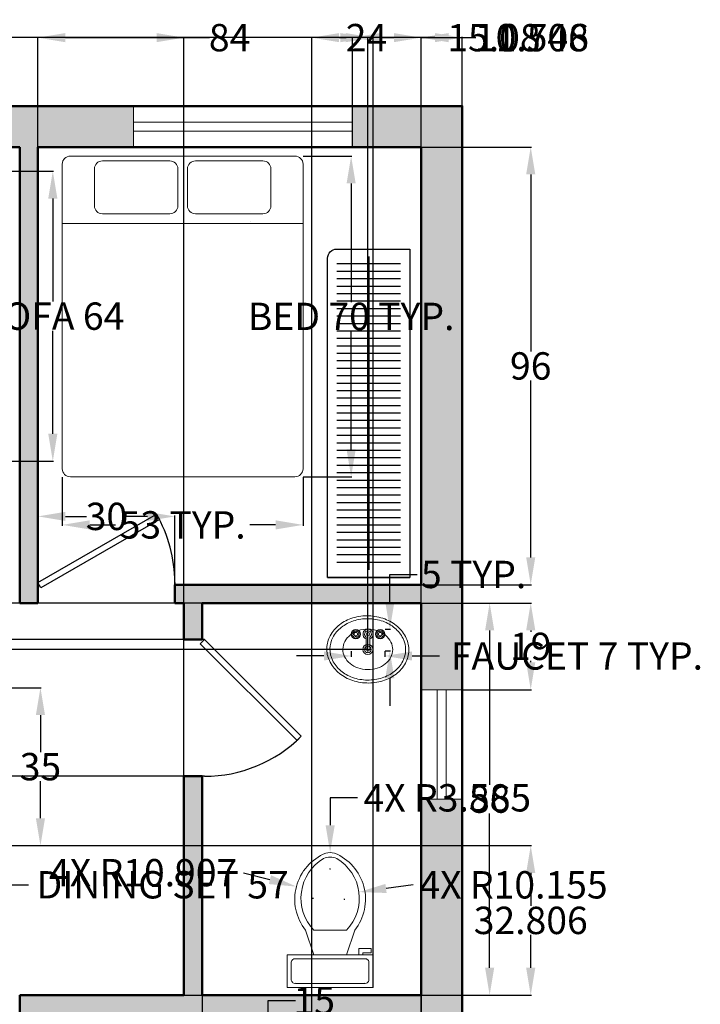
# Model space of a CAD drawing. Units: inches. Extents: x -11 to 341, y -300 to 41.
# Tile 5 of 5: x 192 to 341, y -178 to 38. Entities that reach past the tile are written whole.
import ezdxf

# ---------------------------------------------------------------- set-up
doc = ezdxf.new("R2010")
doc.units = ezdxf.units.IN
doc.header["$MEASUREMENT"] = 0
for name, color, linetype, lineweight in [('A-ANNO-DIMS', 2, 'Continuous', 18), ('A-DOOR', 3, 'Continuous', 25), ('A-FLOR-CASE', 8, 'Continuous', 25), ('A-FLOR-FIXT', 9, 'Continuous', 18), ('A-FURN', 8, 'Continuous', 18), ('A-GLAZ', 4, 'Continuous', 18), ('A-WALL', 7, 'Continuous', 50), ('A-WALL-PATT', 251, 'Continuous', 13)]:
    doc.layers.add(name, color=color, linetype=linetype, lineweight=lineweight)
doc.styles.get("Standard").update_dxf_attribs({"font": 'arial.ttf'})
doc.dimstyles.get("Standard").update_dxf_attribs({"dimtxt": 6, "dimasz": 6, "dimexe": 0.18, "dimexo": 0.0625, "dimgap": 0.09, "dimtad": 0, "dimtih": 1, "dimtoh": 1, "dimdec": 0, "dimzin": 0, "dimdsep": 46, "dimlunit": 4, "dimtxsty": 'Standard', "dimcen": 0.09, "dimadec": 0, "dimazin": 0, "dimtfac": 1, "dimtdec": 0, "dimtofl": 0, "dimtmove": 0, "dimatfit": 3, "dimfxl": 1, "dimtolj": 1, "dimtzin": 0, "dimarcsym": 0})

# ---------------------------------------------------------------- blocks, each defined once
blk = doc.blocks.new('*U2')
for p, q in [((0, 0), (0, -6)), ((40, 0), (40, -6))]:
    blk.add_line(p, q)
blk.add_lwpolyline([(0, 0), (34.64, 20), (35.52, 18.48), (0.87, -1.52)], close=True)
blk.add_arc((0, 0), 40, 0, 30)
blk = doc.blocks.new('*U14')
for p, q in [((0, 0), (0, -6)), ((40, 0), (40, -6))]:
    blk.add_line(p, q)
blk.add_lwpolyline([(0, 0), (28.28, 28.28), (29.52, 27.05), (1.24, -1.24)], close=True)
blk.add_arc((0, 0), 40, 0, 45)
blk = doc.blocks.new('Bed - Queen')
for p, q in [((2, 0), (57.99999, 0)), ((0, -78.00003), (0, -2)), ((9.99999, -1.2), (26.79998, -1.2)), ((33.19999, -1.2), (49.99999, -1.2)), ((59.99999, -2), (59.99999, -78.00003)), ((7.99999, -12.4), (7.99999, -3.2)), ((28.79998, -3.2), (28.79998, -12.4)), ((31.19999, -12.4), (31.19999, -3.2)), ((51.99999, -3.2), (51.99999, -12.4)), ((9.99999, -14.4), (26.79998, -14.4)), ((33.19999, -14.4), (49.99999, -14.4)), ((59.99999, -16.8), (0, -16.8)), ((46.8, -16.4), (46.79936, -16.4)), ((57.99999, -80.00003), (2, -80.00003))]:
    blk.add_line(p, q)
for centre, start, end in [((2, -2), 90, 180), ((57.99999, -2), 0, 90), ((9.99999, -3.2), 90, 180), ((26.79998, -3.2), 0, 90), ((33.19999, -3.2), 90, 180), ((49.99999, -3.2), 0, 90), ((9.99999, -12.4), 180, 270), ((26.79998, -12.4), 270, 0), ((33.19999, -12.4), 180, 270), ((49.99999, -12.4), 270, 0), ((2, -78.00003), 180, 270), ((57.99999, -78.00003), 270, 0)]:
    blk.add_arc(centre, 2, start, end)
blk = doc.blocks.new('Toilet - top')
for p, q in [((9.5, -6), (9.5, -2)), ((-10, -8.5), (-8, -8.5)), ((-10, -9.5), (-10, -8.5)), ((-7, -9.5), (-10, -9.5)), ((-8, -8.5), (-8, -8)), ((-7, -8), (-7, -9.5)), ((-4, -8), (-6, -14)), ((4, -8), (6, -14)), ((4, -14), (-4, -14))]:
    blk.add_line(p, q)
blk.add_lwpolyline([(10.5, -8), (10.5, 0), (-10.5, 0), (-10.5, -8)], close=True)
for points in [[(-9.5, -2), (-9.5, -6)], [(8.5, -1), (-8.5, -1)], [(-8.5, -7), (8.5, -7)]]:
    blk.add_lwpolyline(points)
for centre, radius, start, end in [((-8.62, -1.88), 0.884, 81.8699, 188.1301), ((8.62, -1.88), 0.884, 351.8699, 98.1301), ((-8.62, -6.12), 0.884, 171.8699, 278.1301), ((8.62, -6.12), 0.884, 261.8699, 8.1301), ((3.52, -21.58), 12.17, 141.4691, 247.9714), ((4.2, -21.82), 11.33, 136.3677, 238.9468), ((-3.52, -21.58), 12.17, 292.0284, 38.5307), ((-4.2, -21.82), 11.33, 301.053, 43.6321), ((0, -27.88), 4, 245.7318, 294.2682), ((0, -29), 4, 254.8605, 285.1395)]:
    blk.add_arc(centre, radius, start, end)
blk = doc.blocks.new('Sink - Oval top')
for p, q in [((-1, 0), (1, 0)), ((0, 1), (0, -1))]:
    blk.add_line(p, q)
for points in [[(-12.23, 0.39, 0.117634), (-11.46, -3.36, 0.104469), (-8.88, -6.8, 0.090016), (-5.08, -9.07, 0.08192), (-0.32, -10.02, 0.08192), (4.49, -9.38, 0.090016), (8.42, -7.36, 0.104469), (11.22, -4.09, 0.117634), (12.23, -0.39, 0.117634), (11.46, 3.36, 0.104469), (8.88, 6.8, 0.090016), (5.08, 9.07, 0.08192), (0.32, 10.02, 0.08192), (-4.49, 9.38, 0.090016), (-8.42, 7.36, 0.104469), (-11.22, 4.09, 0.117634)], [(-11.29, 0.16, 0.118622), (-10.52, -3.25, 0.104678), (-8.07, -6.36, 0.089562), (-4.54, -8.37, 0.081185), (-0.13, -9.15, 0.081185), (4.3, -8.49, 0.089562), (7.89, -6.58, 0.104678), (10.42, -3.55, 0.118622), (11.29, -0.16, 0.118622), (10.52, 3.25, 0.104678), (8.07, 6.36, 0.089562), (4.54, 8.37, 0.081185), (0.13, 9.15, 0.081185), (-4.3, 8.49, 0.089562), (-7.89, 6.58, 0.104678), (-10.42, 3.55, 0.118622)], [(-7.42, 0.08, 0.118283), (-6.91, -2.17, 0.104607), (-5.29, -4.21, 0.089718), (-2.97, -5.53, 0.081436), (-0.07, -6.04, 0.081436), (2.84, -5.59, 0.089718), (5.2, -4.33, 0.104607), (6.86, -2.32, 0.118283), (7.42, -0.08, 0.118283), (6.91, 2.17, 0.104607), (5.29, 4.21, 0.089718), (2.97, 5.53, 0.081436), (0.07, 6.04, 0.081436), (-2.84, 5.59, 0.089718), (-5.2, 4.33, 0.104607), (-6.86, 2.32, 0.118283)]]:
    blk.add_lwpolyline(points, format="xyb", close=True)
for radius in [1.5, 1]:
    blk.add_circle((0, 0), radius)
blk = doc.blocks.new('Faucet - Bathroom top')
for p, q in [((-4.107, 0.125), (-4.375, 0.125)), ((-3.75, 0.4788), (-3.75, 0.75)), ((-3.5, 0.482), (-3.5, 0.75)), ((-3.1461, 0.125), (-2.875, 0.125)), ((3.143, 0.125), (2.875, 0.125)), ((3.5, 0.4788), (3.5, 0.75)), ((3.75, 0.482), (3.75, 0.75)), ((4.1039, 0.125), (4.375, 0.125)), ((-4.1039, -0.125), (-4.375, -0.125)), ((-3.75, -0.4821), (-3.75, -0.75)), ((-3.5, -0.4789), (-3.5, -0.75)), ((-3.143, -0.125), (-2.875, -0.125)), ((-0.5, -0.8639), (-0.5, -4.5)), ((0.5, -4.5), (0.5, -0.8631)), ((3.1461, -0.125), (2.875, -0.125)), ((3.5, -0.4821), (3.5, -0.75)), ((3.75, -0.4789), (3.75, -0.75)), ((4.107, -0.125), (4.375, -0.125))]:
    blk.add_line(p, q)
for centre, radius in [((-3.625, 0), 1.375), ((-4.625, 0), 0.2795), ((-3.625, 0), 0.5), ((-3.625, 1), 0.2795), ((-2.625, 0), 0.2795), ((0, 0), 0.5), ((3.625, 0), 1.375), ((2.625, 0), 0.2795), ((3.625, 0), 0.5), ((3.625, 1), 0.2795), ((4.625, 0), 0.2795), ((-3.625, -1), 0.2795), ((3.625, -1), 0.2795)]:
    blk.add_circle(centre, radius)
for centre, radius, start, end in [((-3.625, 0), 1, 105.2407, 164.2093), ((-3.625, 0), 1, 16.44125, 74.07887), ((0, 0), 1.5, 289.6514, 250.3603), ((0, 0), 1, 300.3431, 239.7554), ((3.625, 0), 1, 106.12, 164.0884), ((3.625, 0), 1, 16.23422, 73.90469), ((-3.625, 0), 1, 196.2342, 253.9047), ((-3.625, 0), 1, 286.12, 344.0884), ((3.625, 0), 1, 196.4413, 254.0789), ((3.625, 0), 1, 285.2407, 344.2093), ((0, -4.5), 0.5, 180, 0)]:
    blk.add_arc(centre, radius, start, end)
blk = doc.blocks.new('WIN-48IN')
for p, q in [((0, 0), (0, 9)), ((48, 9), (48, 0)), ((0, 5.5), (48, 5.5)), ((0, 3.5), (48, 3.5))]:
    blk.add_line(p, q)
blk = doc.blocks.new('WIN-24IN')
for p, q in [((0, 24), (9, 24)), ((3.5, 0), (3.5, 24)), ((5.5, 0), (5.5, 24)), ((9, 0), (0, 0))]:
    blk.add_line(p, q)
blk = doc.blocks.new('WARDROBE-HANGING-RAIL')
for p, q in [((14, 67.09), (0, 67.09)), ((7, 68.73), (7, 0)), ((14, 65.45), (0, 65.45)), ((14, 63.82), (0, 63.82)), ((14, 62.18), (0, 62.18)), ((14, 60.55), (0, 60.55)), ((14, 58.91), (0, 58.91)), ((14, 57.27), (0, 57.27)), ((14, 55.64), (0, 55.64)), ((14, 54), (0, 54)), ((14, 52.36), (0, 52.36)), ((14, 50.73), (0, 50.73)), ((14, 49.09), (0, 49.09)), ((14, 47.45), (0, 47.45)), ((14, 45.82), (0, 45.82)), ((14, 44.18), (0, 44.18)), ((14, 42.55), (0, 42.55)), ((14, 40.91), (0, 40.91)), ((14, 39.27), (0, 39.27)), ((14, 37.64), (0, 37.64)), ((14, 36), (0, 36)), ((14, 34.36), (0, 34.36)), ((14, 32.73), (0, 32.73)), ((14, 31.09), (0, 31.09)), ((14, 29.45), (0, 29.45)), ((14, 27.82), (0, 27.82)), ((14, 26.18), (0, 26.18)), ((14, 24.55), (0, 24.55)), ((14, 22.91), (0, 22.91)), ((14, 21.27), (0, 21.27)), ((14, 19.64), (0, 19.64)), ((14, 18), (0, 18)), ((14, 16.36), (0, 16.36)), ((14, 14.73), (0, 14.73)), ((14, 13.09), (0, 13.09)), ((14, 11.45), (0, 11.45)), ((14, 9.82), (0, 9.82)), ((14, 8.18), (0, 8.18)), ((14, 6.55), (0, 6.55)), ((14, 4.91), (0, 4.91)), ((14, 3.27), (0, 3.27)), ((14, 1.64), (0, 1.64))]:
    blk.add_line(p, q)
blk = doc.blocks.new('*D25')
at = {"layer": 'A-ANNO-DIMS', "color": 0, "lineweight": -2, "transparency": 16777216}
for p, q in [((253.72, 8.43), (264.39, 8.43)), ((264.21, 2.43), (264.21, -23.59)), ((264.21, -55.91), (264.21, -29.9)), ((253.72, -61.91), (264.39, -61.91))]:
    blk.add_line(p, q, dxfattribs=at)
at = {"layer": 'A-ANNO-DIMS', "color": 0, "transparency": 16777216}
for points in [[(263.21, 2.43), (265.21, 2.43), (264.21, 8.43)], [(263.21, -55.91), (265.21, -55.91), (264.21, -61.91)]]:
    blk.add_solid(points, dxfattribs=at)
at = {"layer": 'Defpoints', "color": 0, "transparency": 16777216}
for p in [(253.66, 8.43), (264.21, 8.43), (253.66, -61.91)]:
    blk.add_point(p, dxfattribs=at)
at = {"layer": 'A-ANNO-DIMS', "color": 0, "transparency": 16777216, "insert": (264.21, -26.74), "char_height": 6, "attachment_point": 5}
blk.add_mtext('\\A1;BED 70 TYP.', dxfattribs=at)
blk = doc.blocks.new('*D26')
at = {"layer": 'A-ANNO-DIMS', "color": 0, "lineweight": -2, "transparency": 16777216}
for p, q in [((200.9, -61.98), (200.9, -72.64)), ((253.66, -61.98), (253.66, -72.64)), ((206.9, -72.46), (212.59, -72.46)), ((247.66, -72.46), (241.97, -72.46))]:
    blk.add_line(p, q, dxfattribs=at)
at = {"layer": 'A-ANNO-DIMS', "color": 0, "transparency": 16777216}
for points in [[(206.9, -71.46), (206.9, -73.46), (200.9, -72.46)], [(247.66, -71.46), (247.66, -73.46), (253.66, -72.46)]]:
    blk.add_solid(points, dxfattribs=at)
at = {"layer": 'Defpoints', "color": 0, "transparency": 16777216}
for p in [(200.9, -61.91), (253.66, -61.91), (253.66, -72.46)]:
    blk.add_point(p, dxfattribs=at)
at = {"layer": 'A-ANNO-DIMS', "color": 0, "transparency": 16777216, "insert": (227.28, -72.46), "char_height": 6, "attachment_point": 5}
blk.add_mtext('\\A1;53 TYP.', dxfattribs=at)
blk = doc.blocks.new('*D33')
at = {"layer": 'A-ANNO-DIMS', "color": 0, "lineweight": -2, "transparency": 16777216}
for p, q in [((258.23, -101.21), (252.23, -101.21)), ((264.23, -100.17), (264.23, -101.39)), ((271.58, -100.17), (271.58, -101.39)), ((277.58, -101.21), (283.58, -101.21))]:
    blk.add_line(p, q, dxfattribs=at)
at = {"layer": 'A-ANNO-DIMS', "color": 0, "transparency": 16777216}
for points in [[(258.23, -100.21), (258.23, -102.21), (264.23, -101.21)], [(277.58, -100.21), (277.58, -102.21), (271.58, -101.21)]]:
    blk.add_solid(points, dxfattribs=at)
at = {"layer": 'Defpoints', "color": 0, "transparency": 16777216}
for p in [(264.23, -100.11), (271.58, -100.11), (271.58, -101.21)]:
    blk.add_point(p, dxfattribs=at)
at = {"layer": 'A-ANNO-DIMS', "color": 0, "transparency": 16777216, "insert": (313.7, -101.21), "char_height": 6, "attachment_point": 5}
blk.add_mtext('\\A1;FAUCET 7 TYP.', dxfattribs=at)
blk = doc.blocks.new('*D34')
at = {"layer": 'A-ANNO-DIMS', "color": 0, "lineweight": -2, "transparency": 16777216}
for p, q in [((272.69, -89.33), (272.69, -83.33)), ((272.69, -83.33), (278.69, -83.33)), ((271.65, -95.33), (272.87, -95.33)), ((271.65, -100.11), (272.87, -100.11)), ((272.69, -106.11), (272.69, -112.11))]:
    blk.add_line(p, q, dxfattribs=at)
at = {"layer": 'A-ANNO-DIMS', "color": 0, "transparency": 16777216}
for points in [[(271.69, -89.33), (273.69, -89.33), (272.69, -95.33)], [(271.69, -106.11), (273.69, -106.11), (272.69, -100.11)]]:
    blk.add_solid(points, dxfattribs=at)
at = {"layer": 'Defpoints', "color": 0, "transparency": 16777216}
for p in [(271.58, -95.33), (272.69, -95.33), (271.58, -100.11)]:
    blk.add_point(p, dxfattribs=at)
at = {"layer": 'A-ANNO-DIMS', "color": 0, "transparency": 16777216, "insert": (291.05, -83.33), "char_height": 6, "attachment_point": 5}
blk.add_mtext('\\A1;5 TYP.', dxfattribs=at)
blk = doc.blocks.new('*D38')
at = {"layer": 'A-ANNO-DIMS', "color": 0, "lineweight": -2, "transparency": 16777216}
for p, q in [((245.99, -182.78), (245.99, -176.78)), ((245.99, -176.78), (251.99, -176.78)), ((242.07, -182.78), (246.17, -182.78)), ((245.99, -192.25), (245.99, -188.78)), ((242.07, -198.25), (246.17, -198.25))]:
    blk.add_line(p, q, dxfattribs=at)
at = {"layer": 'A-ANNO-DIMS', "color": 0, "transparency": 16777216}
for points in [[(244.99, -188.78), (246.99, -188.78), (245.99, -182.78)], [(244.99, -192.25), (246.99, -192.25), (245.99, -198.25)]]:
    blk.add_solid(points, dxfattribs=at)
at = {"layer": 'Defpoints', "color": 0, "transparency": 16777216}
for p in [(242.01, -182.78), (245.99, -182.78), (242.01, -198.25)]:
    blk.add_point(p, dxfattribs=at)
at = {"layer": 'A-ANNO-DIMS', "color": 0, "transparency": 16777216, "insert": (256.12, -176.78), "char_height": 6, "attachment_point": 5}
blk.add_mtext('\\A1;15', dxfattribs=at)
blk = doc.blocks.new('*D41')
at = {"layer": 'A-ANNO-DIMS', "color": 0, "lineweight": -2, "transparency": 16777216}
for p, q in [((189.35, 5.11), (199, 5.11)), ((198.82, -0.89), (198.82, -23.48)), ((198.82, -52.47), (198.82, -29.87)), ((189.35, -58.47), (199, -58.47))]:
    blk.add_line(p, q, dxfattribs=at)
at = {"layer": 'A-ANNO-DIMS', "color": 0, "transparency": 16777216}
for points in [[(197.82, -0.89), (199.82, -0.89), (198.82, 5.11)], [(197.82, -52.47), (199.82, -52.47), (198.82, -58.47)]]:
    blk.add_solid(points, dxfattribs=at)
at = {"layer": 'Defpoints', "color": 0, "transparency": 16777216}
for p in [(189.29, 5.11), (198.82, 5.11), (189.29, -58.47)]:
    blk.add_point(p, dxfattribs=at)
at = {"layer": 'A-ANNO-DIMS', "color": 0, "transparency": 16777216, "insert": (198.82, -26.68), "char_height": 6, "attachment_point": 5}
blk.add_mtext('\\A1;SOFA 64', dxfattribs=at)
blk = doc.blocks.new('*D43')
at = {"layer": 'A-ANNO-DIMS', "color": 0, "lineweight": -2, "transparency": 16777216}
for p, q in [((130.2, -142.86), (130.2, -151.57)), ((187.51, -142.86), (187.51, -151.57)), ((136.2, -151.39), (181.51, -151.39)), ((187.51, -151.39), (193.51, -151.39))]:
    blk.add_line(p, q, dxfattribs=at)
at = {"layer": 'A-ANNO-DIMS', "color": 0, "transparency": 16777216}
for points in [[(136.2, -150.39), (136.2, -152.39), (130.2, -151.39)], [(181.51, -150.39), (181.51, -152.39), (187.51, -151.39)]]:
    blk.add_solid(points, dxfattribs=at)
at = {"layer": 'Defpoints', "color": 0, "transparency": 16777216}
for p in [(130.2, -142.8), (187.51, -142.8), (187.51, -151.39)]:
    blk.add_point(p, dxfattribs=at)
at = {"layer": 'A-ANNO-DIMS', "color": 0, "transparency": 16777216, "insert": (222.9, -151.39), "char_height": 6, "attachment_point": 5}
blk.add_mtext('\\A1;DINING SET 57', dxfattribs=at)
blk = doc.blocks.new('*D44')
at = {"layer": 'A-ANNO-DIMS', "color": 0, "lineweight": -2, "transparency": 16777216}
for p, q in [((187.57, -108.16), (196.29, -108.16)), ((196.11, -114.16), (196.11, -122.32)), ((196.11, -136.8), (196.11, -128.63)), ((187.57, -142.8), (196.29, -142.8))]:
    blk.add_line(p, q, dxfattribs=at)
at = {"layer": 'A-ANNO-DIMS', "color": 0, "transparency": 16777216}
for points in [[(195.11, -114.16), (197.11, -114.16), (196.11, -108.16)], [(195.11, -136.8), (197.11, -136.8), (196.11, -142.8)]]:
    blk.add_solid(points, dxfattribs=at)
at = {"layer": 'Defpoints', "color": 0, "transparency": 16777216}
for p in [(187.51, -108.16), (196.11, -108.16), (187.51, -142.8)]:
    blk.add_point(p, dxfattribs=at)
at = {"layer": 'A-ANNO-DIMS', "color": 0, "transparency": 16777216, "insert": (196.11, -125.48), "char_height": 6, "attachment_point": 5}
blk.add_mtext('\\A1;35', dxfattribs=at)
blk = doc.blocks.new('*D45')
at = {"layer": 'A-ANNO-DIMS', "color": 0, "lineweight": -2, "transparency": 16777216}
for p, q in [((24.57, 19.46), (24.57, 34.58)), ((288.57, 19.46), (288.57, 34.58)), ((30.57, 34.4), (149.81, 34.4)), ((282.57, 34.4), (163.32, 34.4))]:
    blk.add_line(p, q, dxfattribs=at)
at = {"layer": 'A-ANNO-DIMS', "color": 0, "transparency": 16777216}
for points in [[(30.57, 35.4), (30.57, 33.4), (24.57, 34.4)], [(282.57, 35.4), (282.57, 33.4), (288.57, 34.4)]]:
    blk.add_solid(points, dxfattribs=at)
at = {"layer": 'Defpoints', "color": 0, "transparency": 16777216}
for p in [(288.57, 34.4), (24.57, 19.4), (288.57, 19.4)]:
    blk.add_point(p, dxfattribs=at)
at = {"layer": 'A-ANNO-DIMS', "color": 0, "transparency": 16777216, "insert": (156.57, 34.4), "char_height": 6, "attachment_point": 5}
blk.add_mtext('\\A1;264', dxfattribs=at)
blk = doc.blocks.new('*D49')
at = {"layer": 'A-ANNO-DIMS', "color": 0, "lineweight": -2, "transparency": 16777216}
for p, q in [((264.48, 10.46), (264.48, 34.58)), ((279.57, 10.46), (279.57, 34.58)), ((270.48, 34.4), (273.57, 34.4)), ((279.57, 34.4), (285.57, 34.4))]:
    blk.add_line(p, q, dxfattribs=at)
at = {"layer": 'A-ANNO-DIMS', "color": 0, "transparency": 16777216}
for points in [[(270.48, 35.4), (270.48, 33.4), (264.48, 34.4)], [(273.57, 35.4), (273.57, 33.4), (279.57, 34.4)]]:
    blk.add_solid(points, dxfattribs=at)
at = {"layer": 'Defpoints', "color": 0, "transparency": 16777216}
for p in [(279.57, 34.4), (264.48, 10.4), (279.57, 10.4)]:
    blk.add_point(p, dxfattribs=at)
at = {"layer": 'A-ANNO-DIMS', "color": 0, "transparency": 16777216, "insert": (295.5, 34.4), "char_height": 6, "attachment_point": 5}
blk.add_mtext('\\A1;15.08', dxfattribs=at)
blk = doc.blocks.new('*D57')
at = {"layer": 'A-ANNO-DIMS', "color": 0, "lineweight": -2, "transparency": 16777216}
for p, q in [((195.57, -85.54), (195.57, 34.58)), ((279.57, -85.54), (279.57, 34.58)), ((201.57, 34.4), (233.19, 34.4)), ((273.57, 34.4), (241.94, 34.4))]:
    blk.add_line(p, q, dxfattribs=at)
at = {"layer": 'A-ANNO-DIMS', "color": 0, "transparency": 16777216}
for points in [[(201.57, 35.4), (201.57, 33.4), (195.57, 34.4)], [(273.57, 35.4), (273.57, 33.4), (279.57, 34.4)]]:
    blk.add_solid(points, dxfattribs=at)
at = {"layer": 'Defpoints', "color": 0, "transparency": 16777216}
for p in [(279.57, 34.4), (195.57, -85.6), (279.57, -85.6)]:
    blk.add_point(p, dxfattribs=at)
at = {"layer": 'A-ANNO-DIMS', "color": 0, "transparency": 16777216, "insert": (237.57, 34.4), "char_height": 6, "attachment_point": 5}
blk.add_mtext('\\A1;84', dxfattribs=at)
blk = doc.blocks.new('*D58')
at = {"layer": 'A-ANNO-DIMS', "color": 0, "lineweight": -2, "transparency": 16777216}
for p, q in [((279.63, 10.4), (303.75, 10.4)), ((303.57, 4.4), (303.57, -34.45)), ((303.57, -79.6), (303.57, -40.76)), ((279.63, -85.6), (303.75, -85.6))]:
    blk.add_line(p, q, dxfattribs=at)
at = {"layer": 'A-ANNO-DIMS', "color": 0, "transparency": 16777216}
for points in [[(302.57, 4.4), (304.57, 4.4), (303.57, 10.4)], [(302.57, -79.6), (304.57, -79.6), (303.57, -85.6)]]:
    blk.add_solid(points, dxfattribs=at)
at = {"layer": 'Defpoints', "color": 0, "transparency": 16777216}
for p in [(279.57, 10.4), (303.57, 10.4), (279.57, -85.6)]:
    blk.add_point(p, dxfattribs=at)
at = {"layer": 'A-ANNO-DIMS', "color": 0, "transparency": 16777216, "insert": (303.57, -37.6), "char_height": 6, "attachment_point": 5}
blk.add_mtext('\\A1;96', dxfattribs=at)
blk = doc.blocks.new('*D59')
at = {"layer": 'A-ANNO-DIMS', "color": 0, "lineweight": -2, "transparency": 16777216}
for p, q in [((279.63, -89.6), (294.75, -89.6)), ((294.57, -95.6), (294.57, -129.45)), ((294.57, -169.6), (294.57, -135.76)), ((279.63, -175.6), (294.75, -175.6))]:
    blk.add_line(p, q, dxfattribs=at)
at = {"layer": 'A-ANNO-DIMS', "color": 0, "transparency": 16777216}
for points in [[(293.57, -95.6), (295.57, -95.6), (294.57, -89.6)], [(293.57, -169.6), (295.57, -169.6), (294.57, -175.6)]]:
    blk.add_solid(points, dxfattribs=at)
at = {"layer": 'Defpoints', "color": 0, "transparency": 16777216}
for p in [(279.57, -89.6), (279.57, -175.6), (294.57, -175.6)]:
    blk.add_point(p, dxfattribs=at)
at = {"layer": 'A-ANNO-DIMS', "color": 0, "transparency": 16777216, "insert": (294.57, -132.6), "char_height": 6, "attachment_point": 5}
blk.add_mtext('\\A1;86', dxfattribs=at)
blk = doc.blocks.new('*D62')
at = {"layer": 'A-ANNO-DIMS', "color": 0, "lineweight": -2, "transparency": 16777216}
for p, q in [((85.57, -175.54), (85.57, 34.58)), ((227.57, -175.54), (227.57, 34.58)), ((91.57, 34.4), (150.16, 34.4)), ((221.57, 34.4), (162.97, 34.4))]:
    blk.add_line(p, q, dxfattribs=at)
at = {"layer": 'A-ANNO-DIMS', "color": 0, "transparency": 16777216}
for points in [[(91.57, 35.4), (91.57, 33.4), (85.57, 34.4)], [(221.57, 35.4), (221.57, 33.4), (227.57, 34.4)]]:
    blk.add_solid(points, dxfattribs=at)
at = {"layer": 'Defpoints', "color": 0, "transparency": 16777216}
for p in [(227.57, 34.4), (85.57, -175.6), (227.57, -175.6)]:
    blk.add_point(p, dxfattribs=at)
at = {"layer": 'A-ANNO-DIMS', "color": 0, "transparency": 16777216, "insert": (156.57, 34.4), "char_height": 6, "attachment_point": 5}
blk.add_mtext('\\A1;142', dxfattribs=at)
blk = doc.blocks.new('*D63')
at = {"layer": 'A-ANNO-DIMS', "color": 0, "lineweight": -2, "transparency": 16777216}
for p, q in [((231.57, -175.67), (231.57, -295.79)), ((279.57, -175.67), (279.57, -295.79)), ((237.57, -295.61), (251.05, -295.61)), ((273.57, -295.61), (260.08, -295.61))]:
    blk.add_line(p, q, dxfattribs=at)
at = {"layer": 'A-ANNO-DIMS', "color": 0, "transparency": 16777216}
for points in [[(237.57, -294.61), (237.57, -296.61), (231.57, -295.61)], [(273.57, -294.61), (273.57, -296.61), (279.57, -295.61)]]:
    blk.add_solid(points, dxfattribs=at)
at = {"layer": 'Defpoints', "color": 0, "transparency": 16777216}
for p in [(231.57, -175.6), (279.57, -175.6), (279.57, -295.61)]:
    blk.add_point(p, dxfattribs=at)
at = {"layer": 'A-ANNO-DIMS', "color": 0, "transparency": 16777216, "insert": (255.57, -295.61), "char_height": 6, "attachment_point": 5}
blk.add_mtext('\\A1;48', dxfattribs=at)
blk = doc.blocks.new('*D65')
at = {"layer": 'A-ANNO-DIMS', "color": 0, "lineweight": -2, "transparency": 16777216}
for p, q in [((279.63, -89.6), (303.75, -89.6)), ((303.57, -95.6), (303.57, -95.95)), ((303.57, -102.6), (303.57, -102.26)), ((288.63, -108.6), (303.75, -108.6))]:
    blk.add_line(p, q, dxfattribs=at)
at = {"layer": 'A-ANNO-DIMS', "color": 0, "transparency": 16777216}
for points in [[(302.57, -95.6), (304.57, -95.6), (303.57, -89.6)], [(302.57, -102.6), (304.57, -102.6), (303.57, -108.6)]]:
    blk.add_solid(points, dxfattribs=at)
at = {"layer": 'Defpoints', "color": 0, "transparency": 16777216}
for p in [(279.57, -89.6), (288.57, -108.6), (303.57, -108.6)]:
    blk.add_point(p, dxfattribs=at)
at = {"layer": 'A-ANNO-DIMS', "color": 0, "transparency": 16777216, "insert": (303.57, -99.1), "char_height": 6, "attachment_point": 5}
blk.add_mtext('\\A1;19', dxfattribs=at)
blk = doc.blocks.new('*D66')
at = {"layer": 'A-ANNO-DIMS', "color": 0, "lineweight": -2, "transparency": 16777216}
for p, q in [((9.563121, -83.603265), (9.563121, -77.603265)), ((231.502621, -89.603265), (9.383121, -89.603265)), ((231.502621, -97.603265), (9.383121, -97.603265)), ((9.563121, -103.603265), (9.563121, -109.603265))]:
    blk.add_line(p, q, dxfattribs=at)
at = {"layer": 'A-ANNO-DIMS', "color": 0, "transparency": 16777216}
for points in [[(8.563121, -83.603265), (10.563121, -83.603265), (9.563121, -89.603265)], [(8.563121, -103.603265), (10.563121, -103.603265), (9.563121, -97.603265)]]:
    blk.add_solid(points, dxfattribs=at)
at = {"layer": 'Defpoints', "color": 0, "transparency": 16777216}
for p in [(231.565121, -89.603265), (9.563121, -97.603265), (231.565121, -97.603265)]:
    blk.add_point(p, dxfattribs=at)
at = {"layer": 'A-ANNO-DIMS', "color": 0, "transparency": 16777216, "insert": (9.563121, -93.603265), "char_height": 6, "attachment_point": 5}
blk.add_mtext('\\A1;8', dxfattribs=at)
blk = doc.blocks.new('*D67')
at = {"layer": 'A-ANNO-DIMS', "color": 0, "lineweight": -2, "transparency": 16777216}
for p, q in [((231.5, -97.6), (9.38, -97.6)), ((9.56, -103.6), (9.56, -109.45)), ((9.56, -121.6), (9.56, -115.76)), ((231.5, -127.6), (9.38, -127.6))]:
    blk.add_line(p, q, dxfattribs=at)
at = {"layer": 'A-ANNO-DIMS', "color": 0, "transparency": 16777216}
for points in [[(8.56, -103.6), (10.56, -103.6), (9.56, -97.6)], [(8.56, -121.6), (10.56, -121.6), (9.56, -127.6)]]:
    blk.add_solid(points, dxfattribs=at)
at = {"layer": 'Defpoints', "color": 0, "transparency": 16777216}
for p in [(9.56, -97.6), (231.57, -97.6), (231.57, -127.6)]:
    blk.add_point(p, dxfattribs=at)
at = {"layer": 'A-ANNO-DIMS', "color": 0, "transparency": 16777216, "insert": (9.56, -112.6), "char_height": 6, "attachment_point": 5}
blk.add_mtext('\\A1;30', dxfattribs=at)
blk = doc.blocks.new('*D69')
at = {"layer": 'A-ANNO-DIMS', "color": 0, "lineweight": -2, "transparency": 16777216}
for p, q in [((195.57, -85.54), (195.57, -70.42)), ((201.57, -70.6), (206.19, -70.6)), ((219.57, -70.6), (214.94, -70.6)), ((225.57, -85.54), (225.57, -70.42))]:
    blk.add_line(p, q, dxfattribs=at)
at = {"layer": 'A-ANNO-DIMS', "color": 0, "transparency": 16777216}
for points in [[(201.57, -69.6), (201.57, -71.6), (195.57, -70.6)], [(219.57, -69.6), (219.57, -71.6), (225.57, -70.6)]]:
    blk.add_solid(points, dxfattribs=at)
at = {"layer": 'Defpoints', "color": 0, "transparency": 16777216}
for p in [(225.57, -70.6), (195.57, -85.6), (225.57, -85.6)]:
    blk.add_point(p, dxfattribs=at)
at = {"layer": 'A-ANNO-DIMS', "color": 0, "transparency": 16777216, "insert": (210.57, -70.6), "char_height": 6, "attachment_point": 5}
blk.add_mtext('\\A1;30', dxfattribs=at)
blk = doc.blocks.new('*D77')
at = {"layer": 'A-ANNO-DIMS', "color": 0, "lineweight": -2, "transparency": 16777216}
for p, q in [((255.57, -233.85), (255.57, 34.58)), ((279.57, -233.85), (279.57, 34.58)), ((261.57, 34.4), (263.14, 34.4)), ((273.57, 34.4), (271.99, 34.4))]:
    blk.add_line(p, q, dxfattribs=at)
at = {"layer": 'A-ANNO-DIMS', "color": 0, "transparency": 16777216}
for points in [[(261.57, 35.4), (261.57, 33.4), (255.57, 34.4)], [(273.57, 35.4), (273.57, 33.4), (279.57, 34.4)]]:
    blk.add_solid(points, dxfattribs=at)
at = {"layer": 'Defpoints', "color": 0, "transparency": 16777216}
for p in [(279.57, 34.4), (255.57, -233.91), (279.57, -233.91)]:
    blk.add_point(p, dxfattribs=at)
at = {"layer": 'A-ANNO-DIMS', "color": 0, "transparency": 16777216, "insert": (267.57, 34.4), "char_height": 6, "attachment_point": 5}
blk.add_mtext('\\A1;24', dxfattribs=at)
blk = doc.blocks.new('*D82')
at = {"layer": 'A-ANNO-DIMS', "color": 0, "lineweight": -2, "transparency": 16777216}
for p, q in [((269.02, -173.84), (269.02, 34.58)), ((279.57, -175.54), (279.57, 34.58)), ((263.02, 34.4), (257.02, 34.4)), ((285.57, 34.4), (291.57, 34.4))]:
    blk.add_line(p, q, dxfattribs=at)
at = {"layer": 'A-ANNO-DIMS', "color": 0, "transparency": 16777216}
for points in [[(263.02, 35.4), (263.02, 33.4), (269.02, 34.4)], [(285.57, 35.4), (285.57, 33.4), (279.57, 34.4)]]:
    blk.add_solid(points, dxfattribs=at)
at = {"layer": 'Defpoints', "color": 0, "transparency": 16777216}
for p in [(279.57, 34.4), (269.02, -173.9), (279.57, -175.6)]:
    blk.add_point(p, dxfattribs=at)
at = {"layer": 'A-ANNO-DIMS', "color": 0, "transparency": 16777216, "insert": (303.82, 34.4), "char_height": 6, "attachment_point": 5}
blk.add_mtext('\\A1;10.546', dxfattribs=at)
blk = doc.blocks.new('*D83')
at = {"layer": 'A-ANNO-DIMS', "color": 0, "lineweight": -2, "transparency": 16777216}
for p, q in [((267.86, -99.7), (267.86, 34.58)), ((279.57, -89.54), (279.57, 34.58)), ((261.86, 34.4), (255.86, 34.4)), ((285.57, 34.4), (291.57, 34.4))]:
    blk.add_line(p, q, dxfattribs=at)
at = {"layer": 'A-ANNO-DIMS', "color": 0, "transparency": 16777216}
for points in [[(261.86, 35.4), (261.86, 33.4), (267.86, 34.4)], [(285.57, 35.4), (285.57, 33.4), (279.57, 34.4)]]:
    blk.add_solid(points, dxfattribs=at)
at = {"layer": 'Defpoints', "color": 0, "transparency": 16777216}
for p in [(279.57, 34.4), (279.57, -89.6), (267.86, -99.77)]:
    blk.add_point(p, dxfattribs=at)
at = {"layer": 'A-ANNO-DIMS', "color": 0, "transparency": 16777216, "insert": (303.83, 34.4), "char_height": 6, "attachment_point": 5}
blk.add_mtext('\\A1;11.708', dxfattribs=at)
blk = doc.blocks.new('*D84')
at = {"layer": 'A-ANNO-DIMS', "color": 0, "lineweight": -2, "transparency": 16777216}
for p, q in [((9.56, -83.6), (9.56, -77.6)), ((279.5, -89.6), (9.38, -89.6)), ((267.79, -99.77), (9.38, -99.77)), ((9.56, -105.77), (9.56, -111.77))]:
    blk.add_line(p, q, dxfattribs=at)
at = {"layer": 'A-ANNO-DIMS', "color": 0, "transparency": 16777216}
for points in [[(8.56, -83.6), (10.56, -83.6), (9.56, -89.6)], [(8.56, -105.77), (10.56, -105.77), (9.56, -99.77)]]:
    blk.add_solid(points, dxfattribs=at)
at = {"layer": 'Defpoints', "color": 0, "transparency": 16777216}
for p in [(9.56, -89.6), (279.57, -89.6), (267.86, -99.77)]:
    blk.add_point(p, dxfattribs=at)
at = {"layer": 'A-ANNO-DIMS', "color": 0, "transparency": 16777216, "insert": (9.56, -94.68), "char_height": 6, "attachment_point": 5}
blk.add_mtext('\\A1;10.163', dxfattribs=at)
blk = doc.blocks.new('*D86')
at = {"layer": 'A-ANNO-DIMS', "color": 0, "lineweight": -2, "transparency": 16777216}
for p, q in [((171.7, -142.8), (303.75, -142.8)), ((303.57, -148.8), (303.57, -156.04)), ((303.57, -169.6), (303.57, -162.36)), ((227.63, -175.6), (303.75, -175.6))]:
    blk.add_line(p, q, dxfattribs=at)
at = {"layer": 'A-ANNO-DIMS', "color": 0, "transparency": 16777216}
for points in [[(302.57, -148.8), (304.57, -148.8), (303.57, -142.8)], [(302.57, -169.6), (304.57, -169.6), (303.57, -175.6)]]:
    blk.add_solid(points, dxfattribs=at)
at = {"layer": 'Defpoints', "color": 0, "transparency": 16777216}
for p in [(171.63, -142.8), (303.57, -142.8), (227.57, -175.6)]:
    blk.add_point(p, dxfattribs=at)
at = {"layer": 'A-ANNO-DIMS', "color": 0, "transparency": 16777216, "insert": (303.57, -159.2), "char_height": 6, "attachment_point": 5}
blk.add_mtext('\\A1;32.806', dxfattribs=at)
blk = doc.blocks.new('*D87')
at = {"layer": 'A-ANNO-DIMS', "color": 0, "lineweight": -2, "transparency": 16777216}
for p, q in [((240.61, -148.74), (246.41, -150.26)), ((262.67, -154.56), (262.85, -154.56)), ((262.76, -154.65), (262.76, -154.47))]:
    blk.add_line(p, q, dxfattribs=at)
at = {"layer": 'A-ANNO-DIMS', "color": 0, "transparency": 16777216}
blk.add_solid([(246.66, -149.3), (246.16, -151.23), (252.21, -151.79)], dxfattribs=at)
at = {"layer": 'Defpoints', "color": 0, "transparency": 16777216}
for p in [(252.21, -151.79), (262.76, -154.56)]:
    blk.add_point(p, dxfattribs=at)
at = {"layer": 'A-ANNO-DIMS', "color": 0, "transparency": 16777216, "insert": (218.62, -148.74), "char_height": 6, "attachment_point": 5}
blk.add_mtext('\\A1;4X R10.907', dxfattribs=at)
blk = doc.blocks.new('*D88')
at = {"layer": 'A-ANNO-DIMS', "color": 0, "lineweight": -2, "transparency": 16777216}
for p, q in [((277.8, -151.4), (271.85, -152.19)), ((255.75, -154.35), (255.93, -154.35)), ((255.84, -154.44), (255.84, -154.26))]:
    blk.add_line(p, q, dxfattribs=at)
at = {"layer": 'A-ANNO-DIMS', "color": 0, "transparency": 16777216}
blk.add_solid([(271.72, -151.2), (271.99, -153.19), (265.91, -152.99)], dxfattribs=at)
at = {"layer": 'Defpoints', "color": 0, "transparency": 16777216}
for p in [(265.91, -152.99), (255.84, -154.35)]:
    blk.add_point(p, dxfattribs=at)
at = {"layer": 'A-ANNO-DIMS', "color": 0, "transparency": 16777216, "insert": (299.8, -151.4), "char_height": 6, "attachment_point": 5}
blk.add_mtext('\\A1;4X R10.155', dxfattribs=at)
blk = doc.blocks.new('*D89')
at = {"layer": 'A-ANNO-DIMS', "color": 0, "lineweight": -2, "transparency": 16777216}
for p, q in [((265.61, -132.32), (259.61, -132.32)), ((259.61, -132.32), (259.61, -138.32)), ((259.52, -147.91), (259.7, -147.91)), ((259.61, -148), (259.61, -147.82))]:
    blk.add_line(p, q, dxfattribs=at)
at = {"layer": 'A-ANNO-DIMS', "color": 0, "transparency": 16777216}
blk.add_solid([(258.61, -138.32), (260.61, -138.32), (259.61, -144.32)], dxfattribs=at)
at = {"layer": 'Defpoints', "color": 0, "transparency": 16777216}
for p in [(259.61, -144.32), (259.61, -147.91)]:
    blk.add_point(p, dxfattribs=at)
at = {"layer": 'A-ANNO-DIMS', "color": 0, "transparency": 16777216, "insert": (285.28, -132.32), "char_height": 6, "attachment_point": 5}
blk.add_mtext('\\A1;4X R3.585', dxfattribs=at)

msp = doc.modelspace()

# ---------------------------------------------------------------- hatches: boundary and pattern name
at = {"layer": 'A-WALL-PATT'}
h = msp.add_hatch(color=256, dxfattribs=at)
h.dxf.hatch_style = 1
h.paths.add_polyline_path([(216.4841, 19.3967), (182.3924, 19.3967), (182.3924, 10.3967), (191.5651, 10.3967), (191.5651, -89.6033), (195.5651, -89.6033), (195.5651, -85.1033), (195.5651, 10.3967), (216.4841, 10.3967)])
h = msp.add_hatch(color=256, dxfattribs=at)
h.dxf.hatch_style = 1
h.paths.add_polyline_path([(264.4841, 19.3967), (264.4841, 10.3967), (279.5651, 10.3967), (279.5651, -85.6033), (225.5651, -85.6033), (225.5651, -89.6033), (227.5651, -89.6033), (227.5651, -97.6033), (231.5651, -97.6033), (231.5651, -89.6033), (279.5651, -89.6033), (279.5651, -108.6033), (288.5651, -108.6033), (288.5651, 19.3967)])
h = msp.add_hatch(color=256, dxfattribs=at)
h.dxf.hatch_style = 1
h.paths.add_polyline_path([(231.5651, -175.6033), (231.5651, -127.6033), (227.5651, -127.6033), (227.5651, -175.6033), (191.5651, -175.6033), (191.5651, -233.6033), (195.5651, -233.6033), (195.5651, -179.6033), (279.5651, -179.6033), (279.5651, -271.6033), (263.5868, -271.6033), (263.5868, -280.6033), (288.5651, -280.6033), (288.5651, -132.6033), (279.5651, -132.6033), (279.5651, -175.6033)])

# ---------------------------------------------------------------- linework, layer by layer
at = {"layer": 'A-FLOR-CASE'}
msp.add_lwpolyline([(259.0596, -83.9669), (259.0596, -13.9669, -0.41421356), (261.0596, -11.9669), (277.0596, -11.9669), (277.0596, -83.9669), (259.0596, -83.9669), (277.0596, -83.9669)], format="xyb", dxfattribs=at)
at = {"layer": 'A-WALL'}
for p, q in [((117.5651, 10.3967), (191.5651, 10.3967)), ((191.5651, 10.3967), (191.5651, -89.6033)), ((195.5651, 10.3967), (195.5651, -85.6033)), ((195.5651, 10.3967), (279.5651, 10.3967)), ((279.5651, 10.3967), (279.5651, -85.6033)), ((195.5651, -85.6033), (195.5651, -89.6033)), ((225.5651, -85.6033), (279.5651, -85.6033)), ((225.5651, -85.6033), (225.5651, -89.6033)), ((191.5651, -89.6033), (195.5651, -89.6033)), ((225.5651, -89.6033), (227.5651, -89.6033)), ((227.5651, -89.6033), (227.5651, -97.6033)), ((231.5651, -89.6033), (231.5651, -97.6033)), ((231.5651, -89.6033), (279.5651, -89.6033)), ((279.5651, -89.6033), (279.5651, -175.6033)), ((231.5651, -97.6033), (227.5651, -97.6033)), ((231.5651, -127.6033), (227.5651, -127.6033)), ((227.5651, -127.6033), (227.5651, -175.6033)), ((231.5651, -127.6033), (231.5651, -175.6033)), ((227.5651, -175.6033), (191.5651, -175.6033)), ((191.5651, -175.6033), (191.5651, -233.6033)), ((279.5651, -175.6033), (231.5651, -175.6033))]:
    msp.add_line(p, q, dxfattribs=at)
msp.add_lwpolyline([(129.5651, -280.6033), (24.5651, -280.6033), (24.5651, 19.3967), (288.5651, 19.3967), (288.5651, -280.6033), (165.5651, -280.6033)], dxfattribs=at)

# ---------------------------------------------------------------- block references
at = {"layer": 'A-DOOR', "xscale": 0.75, "yscale": 0.75, "zscale": 0.75}
msp.add_blockref('*U2', (195.5651, -85.1033), dxfattribs=at)
at = {"layer": 'A-DOOR', "xscale": 0.75, "yscale": 0.75, "zscale": 0.75, "rotation": 270}
msp.add_blockref('*U14', (232.0651, -97.6033), dxfattribs=at)
at = {"layer": 'A-FLOR-CASE'}
msp.add_blockref('WARDROBE-HANGING-RAIL', (261.0601, -82.3304), dxfattribs=at)
at = {"layer": 'A-FLOR-FIXT', "xscale": 0.7353737338940184, "yscale": 0.7353737338940184, "zscale": 0.7353737338940184}
for name, p in [('Sink - Oval top', (267.8569, -99.7667)), ('Faucet - Bathroom top', (267.9065, -96.4304))]:
    msp.add_blockref(name, p, dxfattribs=at)
at = {"layer": 'A-FLOR-FIXT', "xscale": 0.896325363236769, "yscale": 0.896325363236769, "zscale": 0.896325363236769, "rotation": 180}
msp.add_blockref('Toilet - top', (259.6076, -173.9025), dxfattribs=at)
at = {"layer": 'A-FURN', "xscale": 0.8792308548308669, "yscale": 0.8792308548308669, "zscale": 0.8792308548308669}
msp.add_blockref('Bed - Queen', (200.9045, 8.4257), dxfattribs=at)
at = {"layer": 'A-GLAZ'}
for name, p in [('WIN-48IN', (216.484, 10.397)), ('WIN-24IN', (279.565, -132.603))]:
    msp.add_blockref(name, p, dxfattribs=at)

# ---------------------------------------------------------------- dimensions: what is measured, and where the dimension line sits
at = {"layer": 'A-ANNO-DIMS'}
for base, p1, p2, override, picture, middle in [((288.5651, 34.3987), (24.5651, 19.3967), (288.5651, 19.3967), {"dimdec": 0, "dimlfac": 1, "dimrnd": 0, "dimzin": 0, "dimdsep": 46, "dimlunit": 2}, '*D45', (156.5651, 34.3987)), ((227.5651, 34.3987), (85.5651, -175.6033), (227.5651, -175.6033), {"dimdec": 0, "dimlfac": 1, "dimrnd": 0, "dimzin": 0, "dimdsep": 46, "dimlunit": 2}, '*D62', (156.5651, 34.3987)), ((279.5651, 34.3987), (195.5651, -85.6033), (279.5651, -85.6033), {"dimdec": 0, "dimlfac": 1, "dimrnd": 0, "dimzin": 0, "dimdsep": 46, "dimlunit": 2}, '*D57', (237.5651, 34.3987)), ((279.5651, 34.3987), (255.5651, -233.9102), (279.5651, -233.9102), {"dimdec": 0, "dimlfac": 1, "dimrnd": 0, "dimzin": 0, "dimdsep": 46, "dimlunit": 2}, '*D77', (267.5651, 34.3987)), ((279.5651, 34.3987), (267.8569, -99.7667), (279.5651, -89.6033), {"dimdec": 3, "dimlfac": 1, "dimrnd": 0, "dimzin": 0, "dimdsep": 46, "dimlunit": 2}, '*D83', (303.8332, 34.3987)), ((279.5651, 34.3987), (269.019, -173.9025), (279.5651, -175.6033), {"dimdec": 3, "dimlfac": 1, "dimrnd": 0, "dimzin": 0, "dimdsep": 46, "dimlunit": 2}, '*D82', (303.825, 34.3987)), ((279.5651, 34.3987), (264.4841, 10.3967), (279.5651, 10.3967), {"dimdec": 2, "dimlfac": 1, "dimrnd": 0, "dimzin": 0, "dimdsep": 46, "dimlunit": 2}, '*D49', (295.5023, 34.3987)), ((225.5651, -70.6013), (195.5651, -85.6033), (225.5651, -85.6033), {"dimdec": 0, "dimlfac": 1, "dimrnd": 0, "dimzin": 0, "dimdsep": 46, "dimlunit": 2}, '*D69', (210.5651, -70.6013)), ((279.5651, -295.6053), (231.5651, -175.6033), (279.5651, -175.6033), {"dimdec": 0, "dimlfac": 1, "dimrnd": 0, "dimzin": 0, "dimdsep": 46, "dimlunit": 2}, '*D63', (255.5651, -295.6053))]:
    dim = msp.add_linear_dim(base=base, p1=p1, p2=p2, dimstyle='Standard', override=override, dxfattribs=at)
    dim.commit()
    dim.dimension.update_dxf_attribs({"geometry": picture, "text_midpoint": middle})
for base, p1, p2, angle, override, picture, middle in [((303.5671, 10.3967), (279.5651, -85.6033), (279.5651, 10.3967), 90, {"dimdec": 0, "dimlfac": 1, "dimrnd": 0, "dimzin": 0, "dimdsep": 46, "dimlunit": 2}, '*D58', (303.5671, -37.6033)), ((9.5631, -89.6033), (267.8569, -99.7667), (279.5651, -89.6033), 90, {"dimdec": 3, "dimlfac": 1, "dimrnd": 0, "dimzin": 0, "dimdsep": 46, "dimlunit": 2}, '*D84', (9.5631, -94.685)), ((9.5631, -97.6033), (231.5651, -89.6033), (231.5651, -97.6033), 90, {"dimdec": 0, "dimlfac": 1, "dimrnd": 0, "dimzin": 0, "dimdsep": 46, "dimlunit": 2}, '*D66', (9.5631, -93.6033)), ((294.5671, -175.6033), (279.5651, -89.6033), (279.5651, -175.6033), 270, {"dimdec": 0, "dimlfac": 1, "dimrnd": 0, "dimzin": 0, "dimdsep": 46, "dimlunit": 2}, '*D59', (294.5671, -132.6033)), ((303.5671, -108.6033), (279.5651, -89.6033), (288.5651, -108.6033), 90, {"dimdec": 0, "dimlfac": 1, "dimrnd": 0, "dimzin": 0, "dimdsep": 46, "dimlunit": 2}, '*D65', (303.5671, -99.1033)), ((9.5631, -97.6033), (231.5651, -127.6033), (231.5651, -97.6033), 90, {"dimdec": 0, "dimlfac": 1, "dimrnd": 0, "dimzin": 0, "dimdsep": 46, "dimlunit": 2}, '*D67', (9.5631, -112.6033)), ((196.1081, -108.161), (187.5119, -142.7977), (187.5119, -108.161), 90, {"dimdec": 0, "dimlfac": 1, "dimrnd": 0, "dimzin": 0, "dimdsep": 46, "dimlunit": 2}, '*D44', (196.1081, -125.4794)), ((303.5671, -142.7977), (227.5651, -175.6033), (171.6347, -142.7977), 90, {"dimdec": 3, "dimlfac": 1, "dimrnd": 0, "dimzin": 0, "dimdsep": 46, "dimlunit": 2}, '*D86', (303.5671, -159.2005)), ((245.9904, -182.7778), (242.0123, -198.2482), (242.0123, -182.7778), 90, {"dimdec": 0, "dimlfac": 1, "dimrnd": 0, "dimzin": 0, "dimdsep": 46, "dimlunit": 2}, '*D38', (256.1179, -176.7778))]:
    dim = msp.add_linear_dim(base=base, p1=p1, p2=p2, angle=angle, dimstyle='Standard', override=override, dxfattribs=at)
    dim.commit()
    dim.dimension.update_dxf_attribs({"geometry": picture, "text_midpoint": middle})
for base, p1, p2, text, picture, middle in [((264.2092, 8.4257), (253.6584, -61.9128), (253.6584, 8.4257), 'BED <> TYP.', '*D25', (264.2092, -26.7435)), ((198.8238, 5.1131), (189.2865, -58.4688), (189.2865, 5.1131), 'SOFA <>', '*D41', (198.8238, -26.6778)), ((272.6864, -95.3273), (271.5834, -100.1073), (271.5834, -95.3273), '<> TYP.', '*D34', (291.0486, -83.3273))]:
    dim = msp.add_linear_dim(base=base, p1=p1, p2=p2, angle=90, text=text, dimstyle='Standard', override={"dimdec": 0, "dimlfac": 1, "dimrnd": 0, "dimzin": 0, "dimdsep": 46, "dimlunit": 2}, dxfattribs=at)
    dim.commit()
    dim.dimension.update_dxf_attribs({"geometry": picture, "text_midpoint": middle})
for base, p1, p2, text, picture, middle in [((253.6584, -72.4636), (200.9045, -61.9128), (253.6584, -61.9128), '<> TYP.', '*D26', (227.2815, -72.4636)), ((271.5834, -101.2103), (264.2296, -100.1073), (271.5834, -100.1073), 'FAUCET <> TYP.', '*D33', (313.7041, -101.2103)), ((187.5119, -151.3939), (130.204, -142.7977), (187.5119, -142.7977), 'DINING SET <>', '*D43', (222.898, -151.3939))]:
    dim = msp.add_linear_dim(base=base, p1=p1, p2=p2, text=text, dimstyle='Standard', override={"dimdec": 0, "dimlfac": 1, "dimrnd": 0, "dimzin": 0, "dimdsep": 46, "dimlunit": 2}, dxfattribs=at)
    dim.commit()
    dim.dimension.update_dxf_attribs({"geometry": picture, "text_midpoint": middle})
for center, mpoint, picture, middle in [((259.6076, -147.909), (259.608, -144.3237), '*D89', (285.2833, -132.3237)), ((262.7622, -154.5593), (252.2126, -151.7887), '*D87', (218.624, -148.7405)), ((255.8431, -154.347), (265.9072, -152.994), '*D88', (299.8049, -151.3951))]:
    dim = msp.add_radius_dim(center=center, mpoint=mpoint, text='4X <>', dimstyle='Standard', override={"dimdec": 3, "dimlfac": 1, "dimrnd": 0, "dimzin": 0, "dimdsep": 46, "dimlunit": 2}, dxfattribs=at)
    dim.commit()
    dim.dimension.update_dxf_attribs({"geometry": picture, "text_midpoint": middle})

doc.saveas('drawing.dxf')
